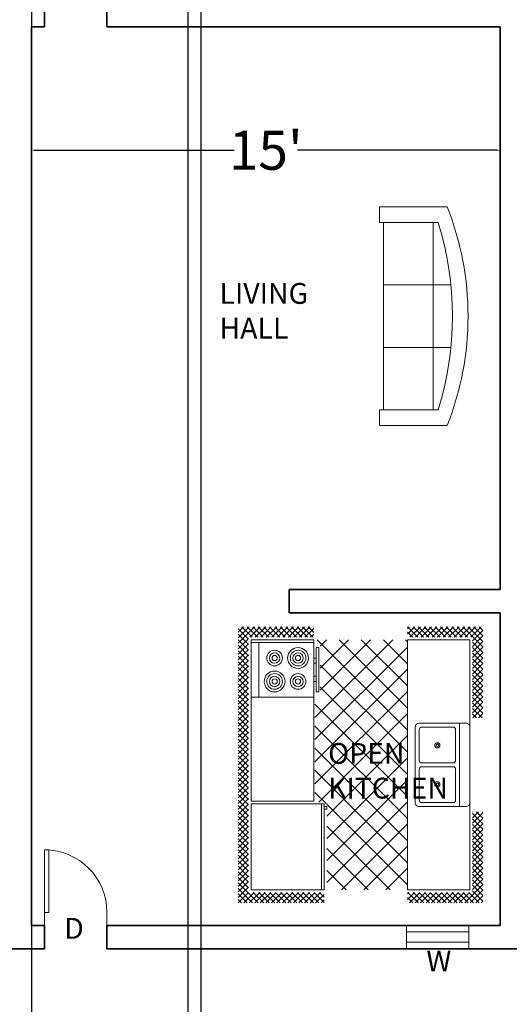
# Model space of a CAD drawing. Units: inches. Extents: x 371 to 1095, y -45 to 1219.
# Tile 10 of 18: x 668 to 856, y 421 to 799. Entities that reach past the tile are written whole.
import ezdxf

# ---------------------------------------------------------------- set-up
doc = ezdxf.new("R2010")
doc.units = ezdxf.units.IN
doc.header["$MEASUREMENT"] = 0
for name, color, linetype, lineweight in [('A-ANNO-DIMS', 2, 'Continuous', 18), ('A-ANNO-TEXT', 7, 'Continuous', 18), ('A-AREA-IDEN', 7, 'Continuous', 18), ('A-DOOR', 3, 'Continuous', 18), ('A-FLOR-FIXT', 9, 'Continuous', 18), ('A-FURN', 254, 'Continuous', 18), ('A-GLAZ', 4, 'Continuous', 18), ('A-WALL', 40, 'Continuous', 35)]:
    doc.layers.add(name, color=color, linetype=linetype, lineweight=lineweight)
doc.styles.get("Standard").update_dxf_attribs({"font": 'arial.ttf'})
doc.dimstyles.get("Standard").update_dxf_attribs({"dimtxt": 1, "dimasz": 1, "dimexe": 0.18, "dimexo": 0.0625, "dimgap": 0.09, "dimtad": 0, "dimtih": 1, "dimtoh": 1, "dimdec": 0, "dimzin": 0, "dimdsep": 46, "dimlunit": 3, "dimtxsty": 'Standard', "dimcen": 0.09, "dimadec": 0, "dimazin": 0, "dimtfac": 1, "dimtdec": 0, "dimtofl": 0, "dimtmove": 0, "dimatfit": 3, "dimfxl": 1, "dimtolj": 1, "dimtzin": 0, "dimarcsym": 0})

# ---------------------------------------------------------------- blocks, each defined once
blk = doc.blocks.new('*U12')
for p, q in [((0, 0), (0, 5)), ((24, 0), (24, 5))]:
    blk.add_line(p, q)
blk.add_lwpolyline([(0, 0), (0, -24), (1.75, -24), (1.75, 0)], close=True)
blk.add_arc((0, 0), 24, 270, 0)
blk = doc.blocks.new('Sofa - Roundback 7 ft.')
for p, q in [((-12.00002, -32.4421), (-12.00003, -6.5971)), ((11.99997, -32.4421), (11.99998, -6.5971)), ((-36.000027, -34), (-36.000027, -11.4696)), ((-35.999844, -13.3819), (35.9998, -13.3819)), ((35.99998, -34), (35.99998, -11.4696)), ((-36.000027, -32.4421), (35.99998, -32.4421))]:
    blk.add_line(p, q)
for points in [[(-36.000027, -34), (-42.000027, -34), (-42.000027, -8)], [(41.99998, -8), (41.99998, -34), (35.99998, -34)]]:
    blk.add_lwpolyline(points)
for centre, radius, start, end in [((0, -114.25), 114.25, 68.43141, 111.5686), ((-0.00001, -127.1968), 121.1968, 72.72033, 107.2797)]:
    blk.add_arc(centre, radius, start, end)
blk = doc.blocks.new('Kitchen Layout - 7 x 8 ft')
for p, q in [((-5, 81.32), (2.68, 89)), ((-5, 83.44), (0.56, 89)), ((-5, 85.56), (-1.56, 89)), ((-5, 87.68), (-3.68, 89)), ((-1, 84.97), (-5, 88.97)), ((1.09, 85), (-2.91, 89)), ((3.21, 85), (-0.79, 89)), ((0.81, 85), (4.81, 89)), ((5.34, 85), (1.34, 89)), ((2.93, 85), (6.93, 89)), ((7.46, 85), (3.46, 89)), ((5.05, 85), (9.05, 89)), ((9.58, 85), (5.58, 89)), ((7.17, 85), (11.17, 89)), ((11.7, 85), (7.7, 89)), ((9.29, 85), (13.29, 89)), ((13.82, 85), (9.82, 89)), ((11.41, 85), (15.41, 89)), ((15.94, 85), (11.94, 89)), ((13.53, 85), (17.53, 89)), ((18.06, 85), (14.06, 89)), ((15.65, 85), (19.65, 89)), ((20.18, 85), (16.18, 89)), ((17.78, 85), (21.78, 89)), ((22.31, 85), (18.31, 89)), ((19.9, 85), (23.9, 89)), ((24.43, 85), (20.43, 89)), ((22.02, 85), (26.02, 89)), ((26.55, 85), (22.55, 89)), ((24.14, 85), (28.14, 89)), ((28.67, 85), (24.67, 89)), ((26.26, 85), (30.26, 89)), ((30.79, 85), (26.79, 89)), ((28.38, 85), (32.38, 89)), ((32.91, 85), (28.91, 89)), ((30.5, 85), (34.5, 89)), ((35.03, 85), (31.03, 89)), ((32.63, 85), (36.63, 89)), ((37.16, 85), (33.16, 89)), ((34.75, 85), (38.75, 89)), ((39.28, 85), (35.28, 89)), ((36.87, 85), (40.87, 89)), ((41.4, 85), (37.4, 89)), ((38.99, 85), (42.99, 89)), ((43.52, 85), (39.52, 89)), ((41.11, 85), (45.11, 89)), ((45.64, 85), (41.64, 89)), ((43.23, 85), (47.23, 89)), ((47.76, 85), (43.76, 89)), ((45.35, 85), (49.35, 89)), ((49.88, 85), (45.88, 89)), ((47.47, 85), (51.47, 89)), ((52, 85), (48, 89)), ((49.6, 85), (53.6, 89)), ((54.13, 85), (50.13, 89)), ((51.72, 85), (55.72, 89)), ((56.25, 85), (52.25, 89)), ((53.84, 85), (57.84, 89)), ((58.37, 85), (54.37, 89)), ((55.96, 85), (59.96, 89)), ((60.49, 85), (56.49, 89)), ((58.08, 85), (62.08, 89)), ((62.61, 85), (58.61, 89)), ((60.2, 85), (64.2, 89)), ((64.73, 85), (60.73, 89)), ((62.32, 85), (66.32, 89)), ((66.85, 85), (62.85, 89)), ((64.45, 85), (68.45, 89)), ((68.97, 85), (64.97, 89)), ((66.57, 85), (70.57, 89)), ((71.1, 85), (67.1, 89)), ((68.69, 85), (72.69, 89)), ((73.22, 85), (69.22, 89)), ((70.81, 85), (74.81, 89)), ((75.34, 85), (71.34, 89)), ((72.93, 85), (76.93, 89)), ((77.46, 85), (73.46, 89)), ((75.05, 85), (79.05, 89)), ((79.58, 85), (75.58, 89)), ((77.17, 85), (81.17, 89)), ((81.7, 85), (77.7, 89)), ((79.29, 85), (83.29, 89)), ((83.82, 85), (79.82, 89)), ((81.42, 85), (85.42, 89)), ((85.95, 85), (81.95, 89)), ((83.54, 85), (87.54, 89)), ((88.07, 85), (84.07, 89)), ((85.66, 85), (89.66, 89)), ((90.19, 85), (86.19, 89)), ((87.78, 85), (91.78, 89)), ((92.31, 85), (88.31, 89)), ((89.9, 85), (93.9, 89)), ((94.43, 85), (90.43, 89)), ((92.02, 85), (96.02, 89)), ((96.55, 85), (92.55, 89)), ((94.14, 85), (98.14, 89)), ((101, 82.67), (94.67, 89)), ((96.27, 85), (100.27, 89)), ((101, 84.79), (96.79, 89)), ((97, 83.61), (101, 87.61)), ((101, 86.92), (98.92, 89)), ((-1, 82.85), (-5, 86.85)), ((-1, 80.73), (-5, 84.73)), ((-5, 79.19), (-1, 83.19)), ((34, 84), (96, 84)), ((34, 60), (34, 84)), ((96, 84), (96, 60)), ((97, 81.49), (101, 85.49)), ((101, 80.55), (97, 84.55)), ((97, 79.37), (101, 83.37)), ((-1, 78.61), (-5, 82.61)), ((-5, 77.07), (-1, 81.07)), ((-1, 76.49), (-5, 80.49)), ((74, 81), (95, 81)), ((101, 78.43), (97, 82.43)), ((97, 77.25), (101, 81.25)), ((101, 76.31), (97, 80.31)), ((-5, 74.95), (-1, 78.95)), ((-1, 74.36), (-5, 78.36)), ((-5, 72.83), (-1, 76.83)), ((-1, 72.24), (-5, 76.24)), ((97, 75.13), (101, 79.13)), ((101, 74.19), (97, 78.19)), ((97, 73.01), (101, 77.01)), ((101, 72.07), (97, 76.07)), ((-5, 70.71), (-1, 74.71)), ((-1, 70.12), (-5, 74.12)), ((-5, 68.59), (-1, 72.59)), ((-1, 68), (-5, 72)), ((97, 70.89), (101, 74.89)), ((101, 69.95), (97, 73.95)), ((97, 68.76), (101, 72.76)), ((101, 67.82), (97, 71.82)), ((-5, 66.47), (-1, 70.47)), ((-1, 65.88), (-5, 69.88)), ((-5, 64.35), (-1, 68.35)), ((97, 66.64), (101, 70.64)), ((101, 65.7), (97, 69.7)), ((97, 64.52), (101, 68.52)), ((-1, 63.76), (-5, 67.76)), ((-5, 62.22), (-1, 66.22)), ((-1, 61.64), (-5, 65.64)), ((101, 63.58), (97, 67.58)), ((97, 62.4), (101, 66.4)), ((101, 61.46), (97, 65.46)), ((97, 60.28), (101, 64.28)), ((-5, 60.1), (-1, 64.1)), ((-1, 59.52), (-5, 63.52)), ((-5, 57.98), (-1, 61.98)), ((-1, 57.39), (-5, 61.39)), ((100.34, 60), (97, 63.34)), ((98.22, 60), (97, 61.22)), ((98.84, 60), (101, 62.16)), ((-1.73, 56), (-5, 59.27)), ((-3.85, 56), (-5, 57.15)), ((-4.86, 56), (-1, 59.86)), ((-2.74, 56), (-1, 57.74)), ((0, 57), (33, 57)), ((10.4, 24), (45.9, 59.5)), ((18.88, 24), (54.38, 59.5)), ((27.37, 24), (62.87, 59.5)), ((33.03, 55.11), (37.41, 59.5)), ((67.71, 24), (33.68, 58.04)), ((96, 60), (34, 60)), ((35.85, 24), (71.35, 59.5)), ((76.2, 24), (40.7, 59.5)), ((44.34, 24), (77.84, 57.5)), ((84.68, 24), (49.18, 59.5)), ((52.82, 24), (86.32, 57.5)), ((93.17, 24), (57.67, 59.5)), ((61.31, 24), (96, 58.69)), ((96, 29.65), (66.15, 59.5)), ((96, 38.14), (76.64, 57.5)), ((80, 60), (80, 59)), ((82, 59), (82, 60)), ((96, 46.63), (85.13, 57.5)), ((87, 59), (87, 60)), ((89, 60), (89, 59)), ((96, 55.11), (93.57, 57.54)), ((100.96, 60), (101, 60.04)), ((0, 30.57), (24.43, 55)), ((0, 39.06), (15.94, 55)), ((0, 47.54), (7.46, 55)), ((1.91, 24), (32.91, 55)), ((33.77, 24), (2.77, 55)), ((42.26, 24), (11.26, 55)), ((50.74, 24), (19.74, 55)), ((59.23, 24), (28.23, 55)), ((31, 55), (31, 56)), ((32, 55), (31, 55)), ((32, 56), (32, 55)), ((25.29, 24), (0, 49.29)), ((69.79, 24), (96, 50.21)), ((78.28, 24), (96, 41.72)), ((16.8, 24), (0, 40.8)), ((8.32, 24), (0, 32.32)), ((86.76, 24), (96, 33.24)), ((-5, 21.92), (-2.92, 24)), ((-5, 19.8), (-1, 23.8)), ((-1, 19.21), (-5, 23.21)), ((-1, 21.33), (-3.67, 24)), ((-1, 23.45), (-1.55, 24)), ((0, 24), (96, 24)), ((0, 0), (0, 24)), ((95.25, 24), (96, 24.75)), ((96, 24), (96, 0)), ((97, 22.1), (98.9, 24)), ((97, 19.97), (101, 23.97)), ((101, 19.03), (97, 23.03)), ((101, 21.16), (98.16, 24)), ((101, 23.28), (100.28, 24)), ((-5, 17.68), (-1, 21.68)), ((-1, 17.09), (-5, 21.09)), ((-5, 15.55), (-1, 19.55)), ((-1, 14.97), (-5, 18.97)), ((97, 17.85), (101, 21.85)), ((101, 16.91), (97, 20.91)), ((97, 15.73), (101, 19.73)), ((-5, 13.43), (-1, 17.43)), ((-1, 12.85), (-5, 16.85)), ((-5, 11.31), (-1, 15.31)), ((47.25, 6.5), (47.25, 18.5)), ((48.75, 18.5), (48.75, 6.5)), ((101, 14.79), (97, 18.79)), ((97, 13.61), (101, 17.61)), ((101, 12.67), (97, 16.67)), ((97, 11.49), (101, 15.49)), ((-1, 10.73), (-5, 14.73)), ((-5, 9.19), (-1, 13.19)), ((-1, 8.6), (-5, 12.6)), ((101, 10.55), (97, 14.55)), ((97, 9.37), (101, 13.37)), ((101, 8.43), (97, 12.43)), ((-5, 7.07), (-1, 11.07)), ((-1, 6.48), (-5, 10.48)), ((-5, 4.95), (-1, 8.95)), ((-1, 4.36), (-5, 8.36)), ((97, 7.25), (101, 11.25)), ((101, 6.31), (97, 10.31)), ((97, 5.12), (101, 9.12)), ((101, 4.18), (97, 8.18)), ((-5, 2.83), (-1, 6.83)), ((-1, 2.24), (-5, 6.24)), ((-5, 0.71), (-1, 4.71)), ((-1, 0.12), (-5, 4.12)), ((64, 4), (32, 4)), ((97, 3), (101, 7)), ((101, 2.06), (97, 6.06)), ((97, 0.88), (101, 4.88)), ((101, -0.06), (97, 3.94)), ((-5, -1.42), (-1, 2.58)), ((2, -5), (-5, 2)), ((-5, -3.54), (-1, 0.46)), ((96, 0), (0, 0)), ((93.24, -5), (101, 2.76)), ((95.36, -5), (101, 0.64)), ((101, -2.18), (97, 1.82)), ((-0.12, -5), (-5, -0.12)), ((-2.25, -5), (-5, -2.25)), ((-4.34, -5), (-0.34, -1)), ((-2.22, -5), (1.78, -1)), ((-0.1, -5), (3.9, -1)), ((4.12, -5), (0.12, -1)), ((2.02, -5), (6.02, -1)), ((6.24, -5), (2.24, -1)), ((4.14, -5), (8.14, -1)), ((8.36, -5), (4.36, -1)), ((6.27, -5), (10.27, -1)), ((10.48, -5), (6.48, -1)), ((8.39, -5), (12.39, -1)), ((12.6, -5), (8.6, -1)), ((10.51, -5), (14.51, -1)), ((14.73, -5), (10.73, -1)), ((12.63, -5), (16.63, -1)), ((16.85, -5), (12.85, -1)), ((14.75, -5), (18.75, -1)), ((18.97, -5), (14.97, -1)), ((16.87, -5), (20.87, -1)), ((21.09, -5), (17.09, -1)), ((18.99, -5), (22.99, -1)), ((23.21, -5), (19.21, -1)), ((21.11, -5), (25.11, -1)), ((25.33, -5), (21.33, -1)), ((23.24, -5), (27.24, -1)), ((27.45, -5), (23.45, -1)), ((25.36, -5), (29.36, -1)), ((29.57, -5), (25.57, -1)), ((27.48, -5), (30, -2.48)), ((30, -3.3), (27.7, -1)), ((30, -1.18), (29.82, -1)), ((66, -2.54), (67.54, -1)), ((66, -4.66), (69.66, -1)), ((69.88, -5), (66, -1.12)), ((67.76, -5), (66, -3.24)), ((67.78, -5), (71.78, -1)), ((72, -5), (68, -1)), ((69.9, -5), (73.9, -1)), ((74.12, -5), (70.12, -1)), ((72.03, -5), (76.03, -1)), ((76.24, -5), (72.24, -1)), ((74.15, -5), (78.15, -1)), ((78.36, -5), (74.36, -1)), ((76.27, -5), (80.27, -1)), ((80.49, -5), (76.49, -1)), ((78.39, -5), (82.39, -1)), ((82.61, -5), (78.61, -1)), ((80.51, -5), (84.51, -1)), ((84.73, -5), (80.73, -1)), ((82.63, -5), (86.63, -1)), ((86.85, -5), (82.85, -1)), ((84.75, -5), (88.75, -1)), ((88.97, -5), (84.97, -1)), ((86.88, -5), (90.88, -1)), ((91.09, -5), (87.09, -1)), ((89, -5), (93, -1)), ((93.21, -5), (89.21, -1)), ((91.12, -5), (95.12, -1)), ((95.34, -5), (91.34, -1)), ((97.46, -5), (93.46, -1)), ((99.58, -5), (95.58, -1)), ((101, -4.3), (97, -0.3)), ((97.48, -5), (101, -1.48)), ((99.6, -5), (101, -3.6)), ((-4.37, -5), (-5, -4.37)), ((29.6, -5), (30, -4.6))]:
    blk.add_line(p, q)
for points in [[(0, 56), (0, 84), (33, 84), (33, 56)], [(74, 60), (74, 84), (95, 84), (95, 60)], [(76, 58), (76, 59), (93, 59), (93, 58)]]:
    blk.add_lwpolyline(points, close=True)
for points in [[(32, 1.5), (32, 19.5)], [(33.5, 21), (62.5, 21)], [(34.5, 19.5), (46.25, 19.5)], [(49.75, 19.5), (61.5, 19.5)], [(64, 19.5), (64, 1.5)], [(33.5, 6.5), (33.5, 18.5)], [(62.5, 18.5), (62.5, 6.5)], [(46.25, 5.5), (34.5, 5.5)], [(61.5, 5.5), (49.75, 5.5)], [(62.5, 0), (33.5, 0)]]:
    blk.add_lwpolyline(points)
for centre, radius in [((80, 75), 4), ((80, 75), 3), ((80, 75), 2), ((80, 75), 1), ((89, 75), 3), ((89, 75), 2), ((89, 75), 1), ((80, 66), 3), ((89, 66), 4), ((89, 66), 3), ((80, 66), 2), ((80, 66), 1), ((89, 66), 2), ((89, 66), 1), ((40.5, 12.5), 1), ((40.5, 12.5), 0.5), ((55.5, 12.5), 1), ((55.5, 12.5), 0.5)]:
    blk.add_circle(centre, radius)
for centre, radius, start, end in [((33.5, 19.5), 1.5, 90, 180), ((34.5, 18.5), 1, 90, 180), ((46.25, 18.5), 1, 0, 90), ((49.75, 18.5), 1, 90, 180), ((61.5, 18.5), 1, 0, 90), ((62.5, 19.5), 1.5, 0, 90), ((34.5, 6.5), 1, 180, 270), ((46.25, 6.5), 1, 270, 0), ((49.75, 6.5), 1, 180, 270), ((61.5, 6.5), 1, 270, 0), ((33.5, 1.5), 1.5, 180, 270), ((62.5, 1.5), 1.5, 270, 0)]:
    blk.add_arc(centre, radius, start, end)
blk = doc.blocks.new('*D23')
at = {"layer": 'A-ANNO-DIMS', "color": 0, "lineweight": -2, "transparency": 16777216}
for p, q in [((672.81, 735.34), (672.81, 748.78)), ((673.81, 748.6), (750.7, 748.6)), ((851.81, 748.6), (774.92, 748.6)), ((852.81, 735.34), (852.81, 748.78))]:
    blk.add_line(p, q, dxfattribs=at)
at = {"layer": 'A-ANNO-DIMS', "color": 0, "transparency": 16777216}
for points in [[(673.81, 748.77), (673.81, 748.43), (672.81, 748.6)], [(851.81, 748.77), (851.81, 748.43), (852.81, 748.6)]]:
    blk.add_solid(points, dxfattribs=at)
at = {"layer": 'Defpoints', "color": 0, "transparency": 16777216}
for p in [(852.81, 748.6), (672.81, 735.28), (852.81, 735.28)]:
    blk.add_point(p, dxfattribs=at)
at = {"layer": 'A-ANNO-DIMS', "color": 0, "transparency": 16777216, "insert": (762.81, 748.6), "char_height": 1, "attachment_point": 5}
blk.add_mtext("\\A1;{\\H15x;15'}", dxfattribs=at)
blk = doc.blocks.new('WIN-24-FRONT')
for p, q in [((0, 6.5), (24, 6.5)), ((0, 2.5), (24, 2.5))]:
    blk.add_line(p, q)
blk.add_lwpolyline([(0, 0), (24, 0), (24, 9), (0, 9)], close=True)
blk = doc.blocks.new('*D54')
at = {"layer": 'A-ANNO-DIMS', "color": 0, "lineweight": -2, "transparency": 16777216}
for p, q in [((672.81, 924.96), (672.81, -43.83)), ((732.81, 924.96), (732.81, -43.83)), ((673.81, -43.65), (701.39, -43.65)), ((731.81, -43.65), (704.23, -43.65))]:
    blk.add_line(p, q, dxfattribs=at)
at = {"layer": 'A-ANNO-DIMS', "color": 0, "transparency": 16777216}
for points in [[(673.81, -43.48), (673.81, -43.82), (672.81, -43.65)], [(731.81, -43.48), (731.81, -43.82), (732.81, -43.65)]]:
    blk.add_solid(points, dxfattribs=at)
at = {"layer": 'Defpoints', "color": 0, "transparency": 16777216}
for p in [(672.81, 925.03), (732.81, 925.03), (732.81, -43.65)]:
    blk.add_point(p, dxfattribs=at)
at = {"layer": 'A-ANNO-DIMS', "color": 0, "transparency": 16777216, "insert": (702.81, -43.65), "char_height": 1, "attachment_point": 5}
blk.add_mtext('\\A1;5\'-0"', dxfattribs=at)
blk = doc.blocks.new('*D57')
at = {"layer": 'A-ANNO-DIMS', "color": 0, "lineweight": -2, "transparency": 16777216}
for p, q in [((732.81, 924.96), (732.81, -43.83)), ((737.81, 919.96), (737.81, -43.83)), ((731.81, -43.65), (730.81, -43.65)), ((738.81, -43.65), (739.81, -43.65))]:
    blk.add_line(p, q, dxfattribs=at)
at = {"layer": 'A-ANNO-DIMS', "color": 0, "transparency": 16777216}
for points in [[(731.81, -43.48), (731.81, -43.82), (732.81, -43.65)], [(738.81, -43.48), (738.81, -43.82), (737.81, -43.65)]]:
    blk.add_solid(points, dxfattribs=at)
at = {"layer": 'Defpoints', "color": 0, "transparency": 16777216}
for p in [(732.81, 925.03), (737.81, 920.03), (732.81, -43.65)]:
    blk.add_point(p, dxfattribs=at)
at = {"layer": 'A-ANNO-DIMS', "color": 0, "transparency": 16777216, "insert": (735.31, -43.65), "char_height": 1, "attachment_point": 5}
blk.add_mtext('\\A1;0\'-5"', dxfattribs=at)

msp = doc.modelspace()

# ---------------------------------------------------------------- linework, layer by layer
at = {"layer": 'A-WALL'}
for p, q in [((677.81, 796.03), (677.81, 805.03)), ((701.81, 805.03), (701.81, 796.03)), ((672.81, 796.03), (677.81, 796.03)), ((672.81, 796.03), (672.81, 451.03)), ((701.81, 796.03), (852.81, 796.03)), ((852.81, 580.03), (852.81, 796.03)), ((771.81, 580.03), (852.81, 580.03)), ((771.81, 571.03), (771.81, 580.03)), ((771.81, 571.03), (852.81, 571.03)), ((852.81, 451.03), (852.81, 571.03)), ((672.81, 451.03), (677.81, 451.03)), ((677.81, 442.02), (677.81, 451.03)), ((701.81, 451.03), (701.81, 442.02)), ((701.81, 451.03), (852.81, 451.03)), ((663.81, 442.02), (677.81, 442.02)), ((701.81, 442.02), (852.81, 442.02)), ((852.81, 442.02), (866.81, 442.02))]:
    msp.add_line(p, q, dxfattribs=at)

# ---------------------------------------------------------------- block references
at = {"layer": 'A-DOOR', "xscale": -1, "rotation": 180}
msp.add_blockref('*U12', (677.81, 456.03), dxfattribs=at)
at = {"layer": 'A-FLOR-FIXT', "rotation": 89.99999999999999}
msp.add_blockref('Kitchen Layout - 7 x 8 ft', (841.19, 464.66), dxfattribs=at)
at = {"layer": 'A-FURN', "rotation": 270}
msp.add_blockref('Sofa - Roundback 7 ft.', (840.46, 684.9), dxfattribs=at)
at = {"layer": 'A-GLAZ'}
msp.add_blockref('WIN-24-FRONT', (816.81, 442.02), dxfattribs=at)

# ---------------------------------------------------------------- texts
at = {"layer": 'A-ANNO-TEXT', "char_height": 8, "attachment_point": 1}
for s, insert in [('D', (685.41, 453.87)), ('W', (824.46, 441.37))]:
    msp.add_mtext_dynamic_manual_height_columns(s, width=17.4938, gutter_width=1, heights=[0], dxfattribs=dict(at, insert=insert))
at = {"layer": 'A-AREA-IDEN', "char_height": 8, "attachment_point": 1}
for s, insert in [('LIVING HALL', (745.05, 697.64)), ('OPEN KITCHEN ', (786.73, 521.05))]:
    msp.add_mtext_dynamic_manual_height_columns(s, width=53.6318, gutter_width=1, heights=[0], dxfattribs=dict(at, insert=insert))

# ---------------------------------------------------------------- dimensions: what is measured, and where the dimension line sits
at = {"layer": 'A-ANNO-DIMS'}
for p1, picture, middle in [((672.81, 925.03), '*D54', (702.81, -43.65)), ((737.81, 920.03), '*D57', (735.31, -43.65))]:
    dim = msp.add_linear_dim(base=(732.81, -43.65), p1=p1, p2=(732.81, 925.03), dimstyle='Standard', override={"dimdec": 1, "dimlfac": 1, "dimrnd": 0, "dimzin": 1, "dimdsep": 46, "dimlunit": 4, "dimfrac": 2}, dxfattribs=at)
    dim.commit()
    dim.dimension.update_dxf_attribs({"geometry": picture, "text_midpoint": middle})
dim = msp.add_linear_dim(base=(852.81, 748.6), p1=(672.81, 735.28), p2=(852.81, 735.28), text='{\\H15x;<>}', dimstyle='Standard', override={"dimclrd": 0, "dimclre": 0, "dimclrt": 0}, dxfattribs=at)
dim.commit()
dim.dimension.update_dxf_attribs({"geometry": '*D23', "text_midpoint": (762.81, 748.6)})

doc.saveas('drawing.dxf')
